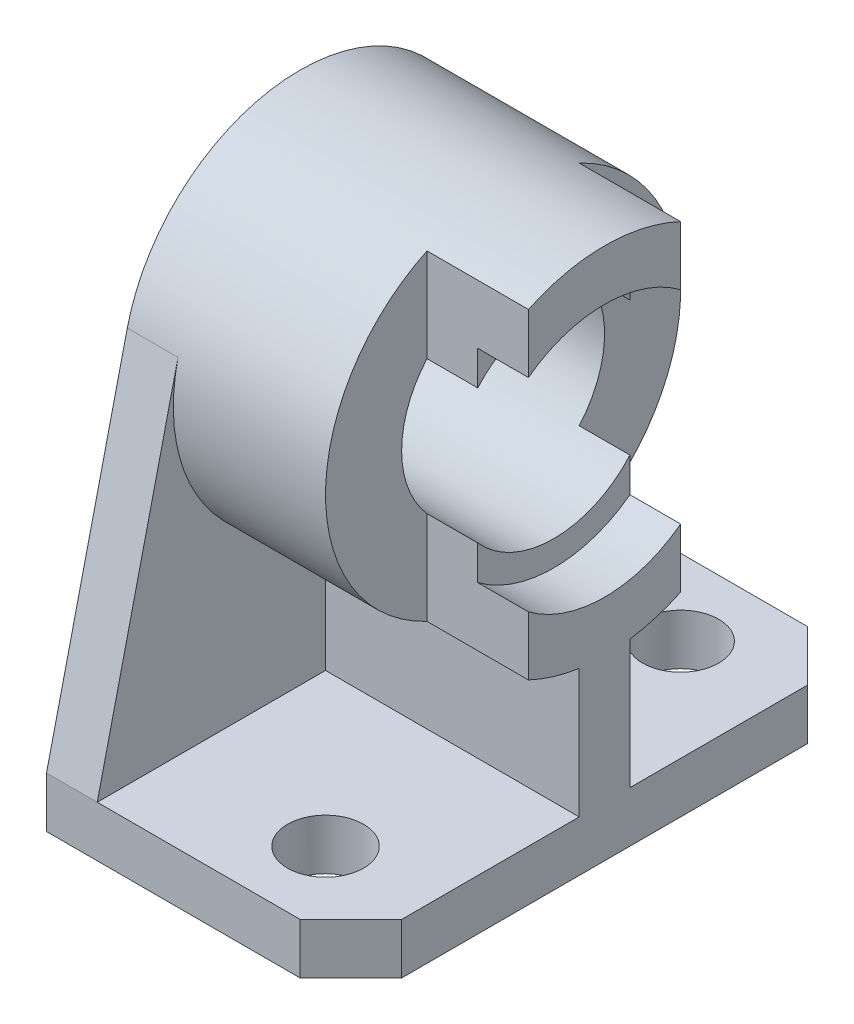
ISO-10303-21;
HEADER;
FILE_DESCRIPTION(('STEP AP214'),'2;1');
FILE_NAME('part.step','',(''),(''),'','','');
FILE_SCHEMA(('AUTOMOTIVE_DESIGN { 1 0 10303 214 1 1 1 1 }'));
ENDSEC;
DATA;
#1=APPLICATION_CONTEXT('core data for automotive mechanical design processes');
#2=APPLICATION_PROTOCOL_DEFINITION('international standard','automotive_design',2000,#1);
#3=PRODUCT_CONTEXT('',#1,'mechanical');
#4=PRODUCT('Part','Part','',(#3));
#5=PRODUCT_RELATED_PRODUCT_CATEGORY('part','',(#4));
#6=PRODUCT_DEFINITION_FORMATION('','',#4);
#7=PRODUCT_DEFINITION_CONTEXT('part definition',#1,'design');
#8=PRODUCT_DEFINITION('design','',#6,#7);
#9=PRODUCT_DEFINITION_SHAPE('','',#8);
#10=(LENGTH_UNIT() NAMED_UNIT(*) SI_UNIT(.MILLI.,.METRE.));
#11=(NAMED_UNIT(*) PLANE_ANGLE_UNIT() SI_UNIT($,.RADIAN.));
#12=(NAMED_UNIT(*) SI_UNIT($,.STERADIAN.) SOLID_ANGLE_UNIT());
#13=UNCERTAINTY_MEASURE_WITH_UNIT(LENGTH_MEASURE(1.E-05),#10,'distance_accuracy_value','');
#14=(GEOMETRIC_REPRESENTATION_CONTEXT(3) GLOBAL_UNCERTAINTY_ASSIGNED_CONTEXT((#13)) GLOBAL_UNIT_ASSIGNED_CONTEXT((#10,
#11,#12)) REPRESENTATION_CONTEXT('',''));
#15=CARTESIAN_POINT('',(0.,0.,0.));
#16=DIRECTION('',(0.,0.,1.));
#17=DIRECTION('',(1.,0.,0.));
#18=AXIS2_PLACEMENT_3D('',#15,#16,#17);
#19=CARTESIAN_POINT('',(60.,-60.,40.));
#20=DIRECTION('',(1.,0.,0.));
#21=DIRECTION('',(0.,0.,-1.));
#22=AXIS2_PLACEMENT_3D('',#19,#20,#21);
#23=PLANE('',#22);
#24=DIRECTION('',(0.,1.,0.));
#25=VECTOR('',#24,1.);
#26=CARTESIAN_POINT('',(60.,31.6227766016838,15.));
#27=LINE('',#26,#25);
#28=CARTESIAN_POINT('',(60.,-31.6227766016838,15.));
#29=VERTEX_POINT('',#28);
#30=CARTESIAN_POINT('',(60.,-20.,15.));
#31=VERTEX_POINT('',#30);
#32=EDGE_CURVE('E216',#29,#31,#27,.T.);
#33=ORIENTED_EDGE('',*,*,#32,.F.);
#34=CARTESIAN_POINT('',(60.,0.,0.));
#35=DIRECTION('',(1.,0.,0.));
#36=DIRECTION('',(0.,0.,-1.));
#37=AXIS2_PLACEMENT_3D('',#34,#35,#36);
#38=CIRCLE('',#37,35.);
#39=CARTESIAN_POINT('',(60.,-34.6410161513775,5.));
#40=VERTEX_POINT('',#39);
#41=EDGE_CURVE('E288',#29,#40,#38,.T.);
#42=ORIENTED_EDGE('',*,*,#41,.T.);
#43=DIRECTION('',(0.,-1.,0.));
#44=VECTOR('',#43,1.);
#45=CARTESIAN_POINT('',(60.,-34.6410161513775,5.));
#46=LINE('',#45,#44);
#47=CARTESIAN_POINT('',(60.,-60.,5.));
#48=VERTEX_POINT('',#47);
#49=EDGE_CURVE('E284',#40,#48,#46,.T.);
#50=ORIENTED_EDGE('',*,*,#49,.T.);
#51=DIRECTION('',(0.,0.,1.));
#52=VECTOR('',#51,1.);
#53=CARTESIAN_POINT('',(60.,-60.,40.));
#54=LINE('',#53,#52);
#55=CARTESIAN_POINT('',(60.,-60.,40.));
#56=VERTEX_POINT('',#55);
#57=EDGE_CURVE('E309',#48,#56,#54,.T.);
#58=ORIENTED_EDGE('',*,*,#57,.T.);
#59=DIRECTION('',(0.,-1.,0.));
#60=VECTOR('',#59,1.);
#61=CARTESIAN_POINT('',(60.,-60.,40.));
#62=LINE('',#61,#60);
#63=CARTESIAN_POINT('',(60.,-70.,40.));
#64=VERTEX_POINT('',#63);
#65=EDGE_CURVE('E334',#56,#64,#62,.T.);
#66=ORIENTED_EDGE('',*,*,#65,.T.);
#67=DIRECTION('',(0.,0.,1.));
#68=VECTOR('',#67,1.);
#69=CARTESIAN_POINT('',(60.,-70.,40.));
#70=LINE('',#69,#68);
#71=CARTESIAN_POINT('',(60.,-70.,-40.));
#72=VERTEX_POINT('',#71);
#73=EDGE_CURVE('E323',#72,#64,#70,.T.);
#74=ORIENTED_EDGE('',*,*,#73,.F.);
#75=DIRECTION('',(0.,-1.,0.));
#76=VECTOR('',#75,1.);
#77=CARTESIAN_POINT('',(60.,-60.,-40.));
#78=LINE('',#77,#76);
#79=CARTESIAN_POINT('',(60.,-60.,-40.));
#80=VERTEX_POINT('',#79);
#81=EDGE_CURVE('E333',#80,#72,#78,.T.);
#82=ORIENTED_EDGE('',*,*,#81,.F.);
#83=CARTESIAN_POINT('',(60.,-60.,-5.));
#84=VERTEX_POINT('',#83);
#85=EDGE_CURVE('E313',#80,#84,#54,.T.);
#86=ORIENTED_EDGE('',*,*,#85,.T.);
#87=DIRECTION('',(0.,1.,0.));
#88=VECTOR('',#87,1.);
#89=CARTESIAN_POINT('',(60.,-34.6410161513775,-5.));
#90=LINE('',#89,#88);
#91=CARTESIAN_POINT('',(60.,-34.6410161513775,-5.00000000000001));
#92=VERTEX_POINT('',#91);
#93=EDGE_CURVE('E292',#84,#92,#90,.T.);
#94=ORIENTED_EDGE('',*,*,#93,.T.);
#95=CARTESIAN_POINT('',(60.,-31.6227766016838,-15.));
#96=VERTEX_POINT('',#95);
#97=EDGE_CURVE('E287',#92,#96,#38,.T.);
#98=ORIENTED_EDGE('',*,*,#97,.T.);
#99=DIRECTION('',(0.,-1.,0.));
#100=VECTOR('',#99,1.);
#101=CARTESIAN_POINT('',(60.,31.6227766016838,-15.));
#102=LINE('',#101,#100);
#103=CARTESIAN_POINT('',(60.,-20.,-15.));
#104=VERTEX_POINT('',#103);
#105=EDGE_CURVE('E416',#104,#96,#102,.T.);
#106=ORIENTED_EDGE('',*,*,#105,.F.);
#107=CARTESIAN_POINT('',(60.,0.,0.));
#108=DIRECTION('',(-1.,0.,0.));
#109=DIRECTION('',(0.,0.,1.));
#110=AXIS2_PLACEMENT_3D('',#107,#108,#109);
#111=CIRCLE('',#110,25.);
#112=EDGE_CURVE('E254',#104,#31,#111,.T.);
#113=ORIENTED_EDGE('',*,*,#112,.T.);
#114=EDGE_LOOP('',(#33,#42,#50,#58,#66,#74,#82,#86,#94,#98,#106,#113));
#115=FACE_BOUND('',#114,.T.);
#116=ADVANCED_FACE('F43',(#115),#23,.T.);
#117=CARTESIAN_POINT('',(0.,0.,0.));
#118=DIRECTION('',(-1.,0.,0.));
#119=DIRECTION('',(0.,0.,1.));
#120=AXIS2_PLACEMENT_3D('',#117,#118,#119);
#121=CYLINDRICAL_SURFACE('',#120,25.);
#122=DIRECTION('',(-1.,0.,0.));
#123=VECTOR('',#122,1.);
#124=CARTESIAN_POINT('',(0.,-20.,15.));
#125=LINE('',#124,#123);
#126=CARTESIAN_POINT('',(50.,-20.,15.));
#127=VERTEX_POINT('',#126);
#128=EDGE_CURVE('E242',#31,#127,#125,.T.);
#129=ORIENTED_EDGE('',*,*,#128,.F.);
#130=ORIENTED_EDGE('',*,*,#112,.F.);
#131=DIRECTION('',(-1.,0.,0.));
#132=VECTOR('',#131,1.);
#133=CARTESIAN_POINT('',(0.,-20.,-15.));
#134=LINE('',#133,#132);
#135=CARTESIAN_POINT('',(50.,-20.,-15.));
#136=VERTEX_POINT('',#135);
#137=EDGE_CURVE('E396',#136,#104,#134,.F.);
#138=ORIENTED_EDGE('',*,*,#137,.F.);
#139=CARTESIAN_POINT('',(50.,0.,0.));
#140=DIRECTION('',(-1.,0.,0.));
#141=DIRECTION('',(0.,0.,1.));
#142=AXIS2_PLACEMENT_3D('',#139,#140,#141);
#143=CIRCLE('',#142,25.);
#144=EDGE_CURVE('E253',#136,#127,#143,.T.);
#145=ORIENTED_EDGE('',*,*,#144,.T.);
#146=EDGE_LOOP('',(#129,#130,#138,#145));
#147=FACE_BOUND('',#146,.T.);
#148=ADVANCED_FACE('F429',(#147),#121,.F.);
#149=CARTESIAN_POINT('',(50.,25.,0.));
#150=DIRECTION('',(1.,0.,0.));
#151=DIRECTION('',(0.,0.,-1.));
#152=AXIS2_PLACEMENT_3D('',#149,#150,#151);
#153=PLANE('',#152);
#154=DIRECTION('',(0.,1.,0.));
#155=VECTOR('',#154,1.);
#156=CARTESIAN_POINT('',(50.,25.,15.));
#157=LINE('',#156,#155);
#158=CARTESIAN_POINT('',(50.,-13.228756555323,15.));
#159=VERTEX_POINT('',#158);
#160=EDGE_CURVE('E237',#127,#159,#157,.T.);
#161=ORIENTED_EDGE('',*,*,#160,.F.);
#162=ORIENTED_EDGE('',*,*,#144,.F.);
#163=DIRECTION('',(0.,-1.,0.));
#164=VECTOR('',#163,1.);
#165=CARTESIAN_POINT('',(50.,25.,-15.));
#166=LINE('',#165,#164);
#167=CARTESIAN_POINT('',(50.,-13.228756555323,-15.));
#168=VERTEX_POINT('',#167);
#169=EDGE_CURVE('E402',#168,#136,#166,.T.);
#170=ORIENTED_EDGE('',*,*,#169,.F.);
#171=CARTESIAN_POINT('',(50.,0.,0.));
#172=DIRECTION('',(-1.,0.,0.));
#173=DIRECTION('',(0.,0.,1.));
#174=AXIS2_PLACEMENT_3D('',#171,#172,#173);
#175=CIRCLE('',#174,20.);
#176=EDGE_CURVE('E249',#168,#159,#175,.T.);
#177=ORIENTED_EDGE('',*,*,#176,.T.);
#178=EDGE_LOOP('',(#161,#162,#170,#177));
#179=FACE_BOUND('',#178,.T.);
#180=ADVANCED_FACE('F452',(#179),#153,.T.);
#181=CARTESIAN_POINT('',(10.,0.,0.));
#182=DIRECTION('',(1.,0.,0.));
#183=DIRECTION('',(0.,0.,-1.));
#184=AXIS2_PLACEMENT_3D('',#181,#182,#183);
#185=PLANE('',#184);
#186=CARTESIAN_POINT('',(10.,0.,0.));
#187=DIRECTION('',(1.,0.,0.));
#188=DIRECTION('',(0.,0.,-1.));
#189=AXIS2_PLACEMENT_3D('',#186,#187,#188);
#190=CIRCLE('',#189,35.);
#191=CARTESIAN_POINT('',(10.,-34.6410161513775,-5.00000000000001));
#192=VERTEX_POINT('',#191);
#193=CARTESIAN_POINT('',(10.,7.981491866062,-34.0777902392744));
#194=VERTEX_POINT('',#193);
#195=EDGE_CURVE('E277',#192,#194,#190,.T.);
#196=ORIENTED_EDGE('',*,*,#195,.F.);
#197=DIRECTION('',(0.,1.,0.));
#198=VECTOR('',#197,1.);
#199=CARTESIAN_POINT('',(10.,-34.6410161513775,-5.));
#200=LINE('',#199,#198);
#201=CARTESIAN_POINT('',(10.,-60.,-5.));
#202=VERTEX_POINT('',#201);
#203=EDGE_CURVE('E276',#202,#192,#200,.T.);
#204=ORIENTED_EDGE('',*,*,#203,.F.);
#205=DIRECTION('',(0.,0.,-1.));
#206=VECTOR('',#205,1.);
#207=CARTESIAN_POINT('',(10.,-60.,50.));
#208=LINE('',#207,#206);
#209=CARTESIAN_POINT('',(10.,-60.,-50.));
#210=VERTEX_POINT('',#209);
#211=EDGE_CURVE('E301',#202,#210,#208,.T.);
#212=ORIENTED_EDGE('',*,*,#211,.T.);
#213=DIRECTION('',(0.,0.973651149693554,0.228042624744629));
#214=VECTOR('',#213,1.);
#215=CARTESIAN_POINT('',(10.,7.981491866062,-34.0777902392744));
#216=LINE('',#215,#214);
#217=EDGE_CURVE('E338',#210,#194,#216,.T.);
#218=ORIENTED_EDGE('',*,*,#217,.T.);
#219=EDGE_LOOP('',(#196,#204,#212,#218));
#220=FACE_BOUND('',#219,.T.);
#221=ADVANCED_FACE('F530',(#220),#185,.T.);
#222=DIRECTION('',(0.,-1.,0.));
#223=VECTOR('',#222,1.);
#224=CARTESIAN_POINT('',(10.,-34.6410161513775,5.));
#225=LINE('',#224,#223);
#226=CARTESIAN_POINT('',(10.,-34.6410161513775,5.));
#227=VERTEX_POINT('',#226);
#228=CARTESIAN_POINT('',(10.,-60.,5.));
#229=VERTEX_POINT('',#228);
#230=EDGE_CURVE('E275',#227,#229,#225,.T.);
#231=ORIENTED_EDGE('',*,*,#230,.F.);
#232=CARTESIAN_POINT('',(10.,7.98149186606201,34.0777902392744));
#233=VERTEX_POINT('',#232);
#234=EDGE_CURVE('E279',#233,#227,#190,.T.);
#235=ORIENTED_EDGE('',*,*,#234,.F.);
#236=DIRECTION('',(0.,-0.973651149693554,0.228042624744629));
#237=VECTOR('',#236,1.);
#238=CARTESIAN_POINT('',(10.,-60.,50.));
#239=LINE('',#238,#237);
#240=CARTESIAN_POINT('',(10.,-60.,50.));
#241=VERTEX_POINT('',#240);
#242=EDGE_CURVE('E344',#233,#241,#239,.T.);
#243=ORIENTED_EDGE('',*,*,#242,.T.);
#244=EDGE_CURVE('E300',#241,#229,#208,.T.);
#245=ORIENTED_EDGE('',*,*,#244,.T.);
#246=EDGE_LOOP('',(#231,#235,#243,#245));
#247=FACE_BOUND('',#246,.T.);
#248=ADVANCED_FACE('F487',(#247),#185,.T.);
#249=CARTESIAN_POINT('',(0.,-60.,0.));
#250=DIRECTION('',(0.,-1.,0.));
#251=DIRECTION('',(0.,0.,-1.));
#252=AXIS2_PLACEMENT_3D('',#249,#250,#251);
#253=PLANE('',#252);
#254=CARTESIAN_POINT('',(40.,-60.,-35.));
#255=DIRECTION('',(0.,1.,0.));
#256=DIRECTION('',(0.,0.,1.));
#257=AXIS2_PLACEMENT_3D('',#254,#255,#256);
#258=CIRCLE('',#257,7.5);
#259=CARTESIAN_POINT('',(40.,-60.,-27.5));
#260=VERTEX_POINT('',#259);
#261=EDGE_CURVE('E257',#260,#260,#258,.T.);
#262=ORIENTED_EDGE('',*,*,#261,.F.);
#263=EDGE_LOOP('',(#262));
#264=FACE_BOUND('',#263,.T.);
#265=DIRECTION('',(-1.,0.,0.));
#266=VECTOR('',#265,1.);
#267=CARTESIAN_POINT('',(178.004237212059,-60.,-5.));
#268=LINE('',#267,#266);
#269=EDGE_CURVE('E270',#84,#202,#268,.T.);
#270=ORIENTED_EDGE('',*,*,#269,.F.);
#271=ORIENTED_EDGE('',*,*,#85,.F.);
#272=DIRECTION('',(0.707106781186548,0.,0.707106781186547));
#273=VECTOR('',#272,1.);
#274=CARTESIAN_POINT('',(50.,-60.,-50.));
#275=LINE('',#274,#273);
#276=CARTESIAN_POINT('',(50.,-60.,-50.));
#277=VERTEX_POINT('',#276);
#278=EDGE_CURVE('E307',#277,#80,#275,.T.);
#279=ORIENTED_EDGE('',*,*,#278,.F.);
#280=DIRECTION('',(1.,0.,0.));
#281=VECTOR('',#280,1.);
#282=CARTESIAN_POINT('',(10.,-60.,-50.));
#283=LINE('',#282,#281);
#284=EDGE_CURVE('E305',#210,#277,#283,.T.);
#285=ORIENTED_EDGE('',*,*,#284,.F.);
#286=ORIENTED_EDGE('',*,*,#211,.F.);
#287=EDGE_LOOP('',(#270,#271,#279,#285,#286));
#288=FACE_BOUND('',#287,.T.);
#289=ADVANCED_FACE('F484',(#264,#288),#253,.F.);
#290=CARTESIAN_POINT('',(40.,-60.,35.));
#291=DIRECTION('',(0.,1.,0.));
#292=DIRECTION('',(0.,0.,-1.));
#293=AXIS2_PLACEMENT_3D('',#290,#291,#292);
#294=CIRCLE('',#293,7.5);
#295=CARTESIAN_POINT('',(40.,-60.,27.5));
#296=VERTEX_POINT('',#295);
#297=EDGE_CURVE('E259',#296,#296,#294,.T.);
#298=ORIENTED_EDGE('',*,*,#297,.F.);
#299=EDGE_LOOP('',(#298));
#300=FACE_BOUND('',#299,.T.);
#301=DIRECTION('',(-1.,0.,0.));
#302=VECTOR('',#301,1.);
#303=CARTESIAN_POINT('',(178.004237212059,-60.,5.));
#304=LINE('',#303,#302);
#305=EDGE_CURVE('E273',#48,#229,#304,.T.);
#306=ORIENTED_EDGE('',*,*,#305,.T.);
#307=ORIENTED_EDGE('',*,*,#244,.F.);
#308=DIRECTION('',(-1.,0.,0.));
#309=VECTOR('',#308,1.);
#310=CARTESIAN_POINT('',(10.,-60.,50.));
#311=LINE('',#310,#309);
#312=CARTESIAN_POINT('',(50.,-60.,50.));
#313=VERTEX_POINT('',#312);
#314=EDGE_CURVE('E320',#313,#241,#311,.T.);
#315=ORIENTED_EDGE('',*,*,#314,.F.);
#316=DIRECTION('',(-0.707106781186547,0.,0.707106781186548));
#317=VECTOR('',#316,1.);
#318=CARTESIAN_POINT('',(50.,-60.,50.));
#319=LINE('',#318,#317);
#320=EDGE_CURVE('E314',#56,#313,#319,.T.);
#321=ORIENTED_EDGE('',*,*,#320,.F.);
#322=ORIENTED_EDGE('',*,*,#57,.F.);
#323=EDGE_LOOP('',(#306,#307,#315,#321,#322));
#324=FACE_BOUND('',#323,.T.);
#325=ADVANCED_FACE('F488',(#300,#324),#253,.F.);
#326=CARTESIAN_POINT('',(10.,-70.,50.));
#327=DIRECTION('',(0.,0.,-1.));
#328=DIRECTION('',(-1.,0.,0.));
#329=AXIS2_PLACEMENT_3D('',#326,#327,#328);
#330=PLANE('',#329);
#331=DIRECTION('',(0.,-1.,0.));
#332=VECTOR('',#331,1.);
#333=CARTESIAN_POINT('',(0.,-70.,50.));
#334=LINE('',#333,#332);
#335=CARTESIAN_POINT('',(0.,-60.,50.));
#336=VERTEX_POINT('',#335);
#337=CARTESIAN_POINT('',(0.,-70.,50.));
#338=VERTEX_POINT('',#337);
#339=EDGE_CURVE('E335',#336,#338,#334,.T.);
#340=ORIENTED_EDGE('',*,*,#339,.T.);
#341=DIRECTION('',(-1.,0.,0.));
#342=VECTOR('',#341,1.);
#343=CARTESIAN_POINT('',(10.,-70.,50.));
#344=LINE('',#343,#342);
#345=CARTESIAN_POINT('',(50.,-70.,50.));
#346=VERTEX_POINT('',#345);
#347=EDGE_CURVE('E375',#346,#338,#344,.T.);
#348=ORIENTED_EDGE('',*,*,#347,.F.);
#349=DIRECTION('',(0.,-1.,0.));
#350=VECTOR('',#349,1.);
#351=CARTESIAN_POINT('',(50.,-60.,50.));
#352=LINE('',#351,#350);
#353=EDGE_CURVE('E328',#313,#346,#352,.T.);
#354=ORIENTED_EDGE('',*,*,#353,.F.);
#355=ORIENTED_EDGE('',*,*,#314,.T.);
#356=DIRECTION('',(-1.,0.,0.));
#357=VECTOR('',#356,1.);
#358=CARTESIAN_POINT('',(10.,-60.,50.));
#359=LINE('',#358,#357);
#360=EDGE_CURVE('E347',#241,#336,#359,.T.);
#361=ORIENTED_EDGE('',*,*,#360,.T.);
#362=EDGE_LOOP('',(#340,#348,#354,#355,#361));
#363=FACE_BOUND('',#362,.T.);
#364=ADVANCED_FACE('F44',(#363),#330,.F.);
#365=CARTESIAN_POINT('',(10.,-70.,50.));
#366=DIRECTION('',(0.,1.,0.));
#367=DIRECTION('',(0.,0.,1.));
#368=AXIS2_PLACEMENT_3D('',#365,#366,#367);
#369=PLANE('',#368);
#370=CARTESIAN_POINT('',(40.,-70.,-35.));
#371=DIRECTION('',(0.,1.,0.));
#372=DIRECTION('',(0.,0.,1.));
#373=AXIS2_PLACEMENT_3D('',#370,#371,#372);
#374=CIRCLE('',#373,7.5);
#375=CARTESIAN_POINT('',(40.,-70.,-27.5));
#376=VERTEX_POINT('',#375);
#377=EDGE_CURVE('E263',#376,#376,#374,.F.);
#378=ORIENTED_EDGE('',*,*,#377,.F.);
#379=EDGE_LOOP('',(#378));
#380=FACE_BOUND('',#379,.T.);
#381=CARTESIAN_POINT('',(40.,-70.,35.));
#382=DIRECTION('',(0.,1.,0.));
#383=DIRECTION('',(0.,0.,1.));
#384=AXIS2_PLACEMENT_3D('',#381,#382,#383);
#385=CIRCLE('',#384,7.5);
#386=CARTESIAN_POINT('',(40.,-70.,42.5));
#387=VERTEX_POINT('',#386);
#388=EDGE_CURVE('E262',#387,#387,#385,.F.);
#389=ORIENTED_EDGE('',*,*,#388,.F.);
#390=EDGE_LOOP('',(#389));
#391=FACE_BOUND('',#390,.T.);
#392=DIRECTION('',(0.,0.,-1.));
#393=VECTOR('',#392,1.);
#394=CARTESIAN_POINT('',(0.,-70.,50.));
#395=LINE('',#394,#393);
#396=CARTESIAN_POINT('',(0.,-70.,-50.));
#397=VERTEX_POINT('',#396);
#398=EDGE_CURVE('E349',#338,#397,#395,.T.);
#399=ORIENTED_EDGE('',*,*,#398,.T.);
#400=DIRECTION('',(-1.,0.,0.));
#401=VECTOR('',#400,1.);
#402=CARTESIAN_POINT('',(10.,-70.,-50.));
#403=LINE('',#402,#401);
#404=CARTESIAN_POINT('',(50.,-70.,-50.));
#405=VERTEX_POINT('',#404);
#406=EDGE_CURVE('E369',#405,#397,#403,.T.);
#407=ORIENTED_EDGE('',*,*,#406,.F.);
#408=DIRECTION('',(0.707106781186548,0.,0.707106781186547));
#409=VECTOR('',#408,1.);
#410=CARTESIAN_POINT('',(50.,-70.,-50.));
#411=LINE('',#410,#409);
#412=EDGE_CURVE('E285',#405,#72,#411,.T.);
#413=ORIENTED_EDGE('',*,*,#412,.T.);
#414=ORIENTED_EDGE('',*,*,#73,.T.);
#415=DIRECTION('',(-0.707106781186547,0.,0.707106781186548));
#416=VECTOR('',#415,1.);
#417=CARTESIAN_POINT('',(50.,-70.,50.));
#418=LINE('',#417,#416);
#419=EDGE_CURVE('E326',#64,#346,#418,.T.);
#420=ORIENTED_EDGE('',*,*,#419,.T.);
#421=ORIENTED_EDGE('',*,*,#347,.T.);
#422=EDGE_LOOP('',(#399,#407,#413,#414,#420,#421));
#423=FACE_BOUND('',#422,.T.);
#424=ADVANCED_FACE('F509',(#380,#391,#423),#369,.F.);
#425=CARTESIAN_POINT('',(10.,-60.,-50.));
#426=DIRECTION('',(0.,0.,1.));
#427=DIRECTION('',(1.,0.,0.));
#428=AXIS2_PLACEMENT_3D('',#425,#426,#427);
#429=PLANE('',#428);
#430=DIRECTION('',(0.,1.,0.));
#431=VECTOR('',#430,1.);
#432=CARTESIAN_POINT('',(0.,-60.,-50.));
#433=LINE('',#432,#431);
#434=CARTESIAN_POINT('',(0.,-60.,-50.));
#435=VERTEX_POINT('',#434);
#436=EDGE_CURVE('E351',#397,#435,#433,.T.);
#437=ORIENTED_EDGE('',*,*,#436,.T.);
#438=DIRECTION('',(-1.,0.,0.));
#439=VECTOR('',#438,1.);
#440=CARTESIAN_POINT('',(10.,-60.,-50.));
#441=LINE('',#440,#439);
#442=EDGE_CURVE('E368',#210,#435,#441,.T.);
#443=ORIENTED_EDGE('',*,*,#442,.F.);
#444=ORIENTED_EDGE('',*,*,#284,.T.);
#445=DIRECTION('',(0.,-1.,0.));
#446=VECTOR('',#445,1.);
#447=CARTESIAN_POINT('',(50.,-60.,-50.));
#448=LINE('',#447,#446);
#449=EDGE_CURVE('E319',#277,#405,#448,.T.);
#450=ORIENTED_EDGE('',*,*,#449,.T.);
#451=ORIENTED_EDGE('',*,*,#406,.T.);
#452=EDGE_LOOP('',(#437,#443,#444,#450,#451));
#453=FACE_BOUND('',#452,.T.);
#454=ADVANCED_FACE('F508',(#453),#429,.F.);
#455=CARTESIAN_POINT('',(10.,7.981491866062,-34.0777902392744));
#456=DIRECTION('',(0.,-0.228042624744629,0.973651149693554));
#457=DIRECTION('',(0.,-0.973651149693554,-0.228042624744629));
#458=AXIS2_PLACEMENT_3D('',#455,#456,#457);
#459=PLANE('',#458);
#460=DIRECTION('',(0.,0.973651149693554,0.228042624744629));
#461=VECTOR('',#460,1.);
#462=CARTESIAN_POINT('',(0.,7.981491866062,-34.0777902392744));
#463=LINE('',#462,#461);
#464=CARTESIAN_POINT('',(0.,7.981491866062,-34.0777902392744));
#465=VERTEX_POINT('',#464);
#466=EDGE_CURVE('E354',#435,#465,#463,.T.);
#467=ORIENTED_EDGE('',*,*,#466,.T.);
#468=DIRECTION('',(-1.,0.,0.));
#469=VECTOR('',#468,1.);
#470=CARTESIAN_POINT('',(10.,7.981491866062,-34.0777902392744));
#471=LINE('',#470,#469);
#472=EDGE_CURVE('E361',#194,#465,#471,.T.);
#473=ORIENTED_EDGE('',*,*,#472,.F.);
#474=ORIENTED_EDGE('',*,*,#217,.F.);
#475=ORIENTED_EDGE('',*,*,#442,.T.);
#476=EDGE_LOOP('',(#467,#473,#474,#475));
#477=FACE_BOUND('',#476,.T.);
#478=ADVANCED_FACE('F525',(#477),#459,.F.);
#479=CARTESIAN_POINT('',(10.,0.,0.));
#480=DIRECTION('',(-1.,0.,0.));
#481=DIRECTION('',(0.,0.,1.));
#482=AXIS2_PLACEMENT_3D('',#479,#480,#481);
#483=CYLINDRICAL_SURFACE('',#482,35.);
#484=ORIENTED_EDGE('',*,*,#41,.F.);
#485=DIRECTION('',(1.,0.,0.));
#486=VECTOR('',#485,1.);
#487=CARTESIAN_POINT('',(40.,-31.6227766016838,15.));
#488=LINE('',#487,#486);
#489=CARTESIAN_POINT('',(40.,-31.6227766016838,15.));
#490=VERTEX_POINT('',#489);
#491=EDGE_CURVE('E226',#490,#29,#488,.T.);
#492=ORIENTED_EDGE('',*,*,#491,.F.);
#493=CARTESIAN_POINT('',(40.,0.,0.));
#494=DIRECTION('',(-1.,0.,0.));
#495=DIRECTION('',(0.,0.,1.));
#496=AXIS2_PLACEMENT_3D('',#493,#494,#495);
#497=CIRCLE('',#496,35.);
#498=CARTESIAN_POINT('',(40.,31.6227766016838,15.));
#499=VERTEX_POINT('',#498);
#500=EDGE_CURVE('E211',#490,#499,#497,.T.);
#501=ORIENTED_EDGE('',*,*,#500,.T.);
#502=DIRECTION('',(1.,0.,0.));
#503=VECTOR('',#502,1.);
#504=CARTESIAN_POINT('',(40.,31.6227766016838,15.));
#505=LINE('',#504,#503);
#506=CARTESIAN_POINT('',(60.,31.6227766016838,15.));
#507=VERTEX_POINT('',#506);
#508=EDGE_CURVE('E218',#499,#507,#505,.T.);
#509=ORIENTED_EDGE('',*,*,#508,.T.);
#510=CARTESIAN_POINT('',(60.,31.6227766016838,-15.));
#511=VERTEX_POINT('',#510);
#512=EDGE_CURVE('E286',#511,#507,#38,.T.);
#513=ORIENTED_EDGE('',*,*,#512,.F.);
#514=DIRECTION('',(1.,0.,0.));
#515=VECTOR('',#514,1.);
#516=CARTESIAN_POINT('',(40.,31.6227766016838,-15.));
#517=LINE('',#516,#515);
#518=CARTESIAN_POINT('',(40.,31.6227766016838,-15.));
#519=VERTEX_POINT('',#518);
#520=EDGE_CURVE('E415',#519,#511,#517,.T.);
#521=ORIENTED_EDGE('',*,*,#520,.F.);
#522=CARTESIAN_POINT('',(40.,0.,0.));
#523=DIRECTION('',(1.,0.,0.));
#524=DIRECTION('',(0.,0.,-1.));
#525=AXIS2_PLACEMENT_3D('',#522,#523,#524);
#526=CIRCLE('',#525,35.);
#527=CARTESIAN_POINT('',(40.,-31.6227766016838,-15.));
#528=VERTEX_POINT('',#527);
#529=EDGE_CURVE('E401',#528,#519,#526,.T.);
#530=ORIENTED_EDGE('',*,*,#529,.F.);
#531=DIRECTION('',(1.,0.,0.));
#532=VECTOR('',#531,1.);
#533=CARTESIAN_POINT('',(40.,-31.6227766016838,-15.));
#534=LINE('',#533,#532);
#535=EDGE_CURVE('E410',#528,#96,#534,.T.);
#536=ORIENTED_EDGE('',*,*,#535,.T.);
#537=ORIENTED_EDGE('',*,*,#97,.F.);
#538=DIRECTION('',(-1.,0.,0.));
#539=VECTOR('',#538,1.);
#540=CARTESIAN_POINT('',(178.004237212059,-34.6410161513775,-5.00000000000001));
#541=LINE('',#540,#539);
#542=EDGE_CURVE('E282',#92,#192,#541,.T.);
#543=ORIENTED_EDGE('',*,*,#542,.T.);
#544=ORIENTED_EDGE('',*,*,#195,.T.);
#545=ORIENTED_EDGE('',*,*,#472,.T.);
#546=CARTESIAN_POINT('',(0.,0.,0.));
#547=DIRECTION('',(1.,0.,0.));
#548=DIRECTION('',(0.,0.,-1.));
#549=AXIS2_PLACEMENT_3D('',#546,#547,#548);
#550=CIRCLE('',#549,35.);
#551=CARTESIAN_POINT('',(0.,7.98149186606201,34.0777902392744));
#552=VERTEX_POINT('',#551);
#553=EDGE_CURVE('E355',#465,#552,#550,.T.);
#554=ORIENTED_EDGE('',*,*,#553,.T.);
#555=DIRECTION('',(-1.,0.,0.));
#556=VECTOR('',#555,1.);
#557=CARTESIAN_POINT('',(10.,7.98149186606201,34.0777902392744));
#558=LINE('',#557,#556);
#559=EDGE_CURVE('E358',#233,#552,#558,.T.);
#560=ORIENTED_EDGE('',*,*,#559,.F.);
#561=ORIENTED_EDGE('',*,*,#234,.T.);
#562=DIRECTION('',(-1.,0.,0.));
#563=VECTOR('',#562,1.);
#564=CARTESIAN_POINT('',(178.004237212059,-34.6410161513775,5.));
#565=LINE('',#564,#563);
#566=EDGE_CURVE('E274',#40,#227,#565,.T.);
#567=ORIENTED_EDGE('',*,*,#566,.F.);
#568=EDGE_LOOP('',(#484,#492,#501,#509,#513,#521,#530,#536,#537,#543,#544,#545,#554,#560,#561,#567));
#569=FACE_BOUND('',#568,.T.);
#570=ADVANCED_FACE('F230',(#569),#483,.T.);
#571=CARTESIAN_POINT('',(10.,-60.,50.));
#572=DIRECTION('',(0.,-0.228042624744629,-0.973651149693554));
#573=DIRECTION('',(0.,0.973651149693554,-0.228042624744629));
#574=AXIS2_PLACEMENT_3D('',#571,#572,#573);
#575=PLANE('',#574);
#576=DIRECTION('',(0.,-0.973651149693554,0.228042624744629));
#577=VECTOR('',#576,1.);
#578=CARTESIAN_POINT('',(0.,-60.,50.));
#579=LINE('',#578,#577);
#580=EDGE_CURVE('E345',#552,#336,#579,.T.);
#581=ORIENTED_EDGE('',*,*,#580,.T.);
#582=ORIENTED_EDGE('',*,*,#360,.F.);
#583=ORIENTED_EDGE('',*,*,#242,.F.);
#584=ORIENTED_EDGE('',*,*,#559,.T.);
#585=EDGE_LOOP('',(#581,#582,#583,#584));
#586=FACE_BOUND('',#585,.T.);
#587=ADVANCED_FACE('F477',(#586),#575,.F.);
#588=CARTESIAN_POINT('',(0.,0.,0.));
#589=DIRECTION('',(1.,0.,0.));
#590=DIRECTION('',(0.,0.,-1.));
#591=AXIS2_PLACEMENT_3D('',#588,#589,#590);
#592=PLANE('',#591);
#593=CARTESIAN_POINT('',(0.,0.,0.));
#594=DIRECTION('',(-1.,0.,0.));
#595=DIRECTION('',(0.,0.,1.));
#596=AXIS2_PLACEMENT_3D('',#593,#594,#595);
#597=CIRCLE('',#596,20.);
#598=CARTESIAN_POINT('',(0.,0.,20.));
#599=VERTEX_POINT('',#598);
#600=EDGE_CURVE('E243',#599,#599,#597,.T.);
#601=ORIENTED_EDGE('',*,*,#600,.F.);
#602=EDGE_LOOP('',(#601));
#603=FACE_BOUND('',#602,.T.);
#604=ORIENTED_EDGE('',*,*,#339,.F.);
#605=ORIENTED_EDGE('',*,*,#580,.F.);
#606=ORIENTED_EDGE('',*,*,#553,.F.);
#607=ORIENTED_EDGE('',*,*,#466,.F.);
#608=ORIENTED_EDGE('',*,*,#436,.F.);
#609=ORIENTED_EDGE('',*,*,#398,.F.);
#610=EDGE_LOOP('',(#604,#605,#606,#607,#608,#609));
#611=FACE_BOUND('',#610,.T.);
#612=ADVANCED_FACE('F474',(#603,#611),#592,.F.);
#613=CARTESIAN_POINT('',(50.,-60.,50.));
#614=DIRECTION('',(0.707106781186548,0.,0.707106781186547));
#615=DIRECTION('',(0.707106781186547,0.,-0.707106781186548));
#616=AXIS2_PLACEMENT_3D('',#613,#614,#615);
#617=PLANE('',#616);
#618=ORIENTED_EDGE('',*,*,#419,.F.);
#619=ORIENTED_EDGE('',*,*,#65,.F.);
#620=ORIENTED_EDGE('',*,*,#320,.T.);
#621=ORIENTED_EDGE('',*,*,#353,.T.);
#622=EDGE_LOOP('',(#618,#619,#620,#621));
#623=FACE_BOUND('',#622,.T.);
#624=ADVANCED_FACE('F467',(#623),#617,.T.);
#625=CARTESIAN_POINT('',(60.,20.,15.));
#626=VERTEX_POINT('',#625);
#627=EDGE_CURVE('E225',#626,#507,#27,.T.);
#628=ORIENTED_EDGE('',*,*,#627,.F.);
#629=CARTESIAN_POINT('',(60.,20.,-15.));
#630=VERTEX_POINT('',#629);
#631=EDGE_CURVE('E258',#626,#630,#111,.T.);
#632=ORIENTED_EDGE('',*,*,#631,.T.);
#633=EDGE_CURVE('E413',#511,#630,#102,.T.);
#634=ORIENTED_EDGE('',*,*,#633,.F.);
#635=ORIENTED_EDGE('',*,*,#512,.T.);
#636=EDGE_LOOP('',(#628,#632,#634,#635));
#637=FACE_BOUND('',#636,.T.);
#638=ADVANCED_FACE('F438',(#637),#23,.T.);
#639=CARTESIAN_POINT('',(50.,-60.,-50.));
#640=DIRECTION('',(0.707106781186547,0.,-0.707106781186548));
#641=DIRECTION('',(-0.707106781186548,0.,-0.707106781186547));
#642=AXIS2_PLACEMENT_3D('',#639,#640,#641);
#643=PLANE('',#642);
#644=ORIENTED_EDGE('',*,*,#412,.F.);
#645=ORIENTED_EDGE('',*,*,#449,.F.);
#646=ORIENTED_EDGE('',*,*,#278,.T.);
#647=ORIENTED_EDGE('',*,*,#81,.T.);
#648=EDGE_LOOP('',(#644,#645,#646,#647));
#649=FACE_BOUND('',#648,.T.);
#650=ADVANCED_FACE('F465',(#649),#643,.T.);
#651=CARTESIAN_POINT('',(178.004237212059,-34.6410161513775,-5.));
#652=DIRECTION('',(0.,0.,1.));
#653=DIRECTION('',(0.,-1.,0.));
#654=AXIS2_PLACEMENT_3D('',#651,#652,#653);
#655=PLANE('',#654);
#656=ORIENTED_EDGE('',*,*,#93,.F.);
#657=ORIENTED_EDGE('',*,*,#269,.T.);
#658=ORIENTED_EDGE('',*,*,#203,.T.);
#659=ORIENTED_EDGE('',*,*,#542,.F.);
#660=EDGE_LOOP('',(#656,#657,#658,#659));
#661=FACE_BOUND('',#660,.T.);
#662=ADVANCED_FACE('F472',(#661),#655,.F.);
#663=CARTESIAN_POINT('',(178.004237212059,-34.6410161513775,5.));
#664=DIRECTION('',(0.,0.,-1.));
#665=DIRECTION('',(0.,1.,0.));
#666=AXIS2_PLACEMENT_3D('',#663,#664,#665);
#667=PLANE('',#666);
#668=ORIENTED_EDGE('',*,*,#49,.F.);
#669=ORIENTED_EDGE('',*,*,#566,.T.);
#670=ORIENTED_EDGE('',*,*,#230,.T.);
#671=ORIENTED_EDGE('',*,*,#305,.F.);
#672=EDGE_LOOP('',(#668,#669,#670,#671));
#673=FACE_BOUND('',#672,.T.);
#674=ADVANCED_FACE('F492',(#673),#667,.F.);
#675=CARTESIAN_POINT('',(40.,-70.001,35.));
#676=DIRECTION('',(0.,1.,0.));
#677=DIRECTION('',(0.,0.,1.));
#678=AXIS2_PLACEMENT_3D('',#675,#676,#677);
#679=CYLINDRICAL_SURFACE('',#678,7.5);
#680=ORIENTED_EDGE('',*,*,#297,.T.);
#681=EDGE_LOOP('',(#680));
#682=FACE_BOUND('',#681,.T.);
#683=ORIENTED_EDGE('',*,*,#388,.T.);
#684=EDGE_LOOP('',(#683));
#685=FACE_BOUND('',#684,.T.);
#686=ADVANCED_FACE('F454',(#682,#685),#679,.F.);
#687=CARTESIAN_POINT('',(40.,-70.001,-35.));
#688=DIRECTION('',(0.,1.,0.));
#689=DIRECTION('',(0.,0.,1.));
#690=AXIS2_PLACEMENT_3D('',#687,#688,#689);
#691=CYLINDRICAL_SURFACE('',#690,7.5);
#692=ORIENTED_EDGE('',*,*,#261,.T.);
#693=EDGE_LOOP('',(#692));
#694=FACE_BOUND('',#693,.T.);
#695=ORIENTED_EDGE('',*,*,#377,.T.);
#696=EDGE_LOOP('',(#695));
#697=FACE_BOUND('',#696,.T.);
#698=ADVANCED_FACE('F441',(#694,#697),#691,.F.);
#699=DIRECTION('',(-1.,0.,0.));
#700=VECTOR('',#699,1.);
#701=CARTESIAN_POINT('',(0.,20.,15.));
#702=LINE('',#701,#700);
#703=CARTESIAN_POINT('',(50.,20.,15.));
#704=VERTEX_POINT('',#703);
#705=EDGE_CURVE('E231',#704,#626,#702,.F.);
#706=ORIENTED_EDGE('',*,*,#705,.F.);
#707=CARTESIAN_POINT('',(50.,20.,-15.));
#708=VERTEX_POINT('',#707);
#709=EDGE_CURVE('E252',#704,#708,#143,.T.);
#710=ORIENTED_EDGE('',*,*,#709,.T.);
#711=DIRECTION('',(-1.,0.,0.));
#712=VECTOR('',#711,1.);
#713=CARTESIAN_POINT('',(0.,20.,-15.));
#714=LINE('',#713,#712);
#715=EDGE_CURVE('E234',#630,#708,#714,.T.);
#716=ORIENTED_EDGE('',*,*,#715,.F.);
#717=ORIENTED_EDGE('',*,*,#631,.F.);
#718=EDGE_LOOP('',(#706,#710,#716,#717));
#719=FACE_BOUND('',#718,.T.);
#720=ADVANCED_FACE('F445',(#719),#121,.F.);
#721=CARTESIAN_POINT('',(50.,13.228756555323,15.));
#722=VERTEX_POINT('',#721);
#723=EDGE_CURVE('E232',#722,#704,#157,.T.);
#724=ORIENTED_EDGE('',*,*,#723,.F.);
#725=CARTESIAN_POINT('',(50.,13.228756555323,-15.));
#726=VERTEX_POINT('',#725);
#727=EDGE_CURVE('E250',#722,#726,#175,.T.);
#728=ORIENTED_EDGE('',*,*,#727,.T.);
#729=EDGE_CURVE('E240',#708,#726,#166,.T.);
#730=ORIENTED_EDGE('',*,*,#729,.F.);
#731=ORIENTED_EDGE('',*,*,#709,.F.);
#732=EDGE_LOOP('',(#724,#728,#730,#731));
#733=FACE_BOUND('',#732,.T.);
#734=ADVANCED_FACE('F389',(#733),#153,.T.);
#735=CARTESIAN_POINT('',(0.,0.,0.));
#736=DIRECTION('',(-1.,0.,0.));
#737=DIRECTION('',(0.,0.,1.));
#738=AXIS2_PLACEMENT_3D('',#735,#736,#737);
#739=CYLINDRICAL_SURFACE('',#738,20.);
#740=DIRECTION('',(-1.,0.,0.));
#741=VECTOR('',#740,1.);
#742=CARTESIAN_POINT('',(0.,-13.228756555323,15.));
#743=LINE('',#742,#741);
#744=CARTESIAN_POINT('',(40.,-13.2287565553229,15.));
#745=VERTEX_POINT('',#744);
#746=EDGE_CURVE('E11',#159,#745,#743,.T.);
#747=ORIENTED_EDGE('',*,*,#746,.F.);
#748=ORIENTED_EDGE('',*,*,#176,.F.);
#749=DIRECTION('',(-1.,0.,0.));
#750=VECTOR('',#749,1.);
#751=CARTESIAN_POINT('',(0.,-13.228756555323,-15.));
#752=LINE('',#751,#750);
#753=CARTESIAN_POINT('',(40.,-13.228756555323,-15.));
#754=VERTEX_POINT('',#753);
#755=EDGE_CURVE('E378',#754,#168,#752,.F.);
#756=ORIENTED_EDGE('',*,*,#755,.F.);
#757=CARTESIAN_POINT('',(40.,0.,0.));
#758=DIRECTION('',(1.,0.,0.));
#759=DIRECTION('',(0.,0.,-1.));
#760=AXIS2_PLACEMENT_3D('',#757,#758,#759);
#761=CIRCLE('',#760,20.);
#762=CARTESIAN_POINT('',(40.,13.228756555323,-15.));
#763=VERTEX_POINT('',#762);
#764=EDGE_CURVE('E374',#754,#763,#761,.T.);
#765=ORIENTED_EDGE('',*,*,#764,.T.);
#766=DIRECTION('',(-1.,0.,0.));
#767=VECTOR('',#766,1.);
#768=CARTESIAN_POINT('',(0.,13.228756555323,-15.));
#769=LINE('',#768,#767);
#770=EDGE_CURVE('E379',#726,#763,#769,.T.);
#771=ORIENTED_EDGE('',*,*,#770,.F.);
#772=ORIENTED_EDGE('',*,*,#727,.F.);
#773=DIRECTION('',(-1.,0.,0.));
#774=VECTOR('',#773,1.);
#775=CARTESIAN_POINT('',(0.,13.228756555323,15.));
#776=LINE('',#775,#774);
#777=CARTESIAN_POINT('',(40.,13.2287565553229,15.));
#778=VERTEX_POINT('',#777);
#779=EDGE_CURVE('E51',#778,#722,#776,.F.);
#780=ORIENTED_EDGE('',*,*,#779,.F.);
#781=CARTESIAN_POINT('',(40.,0.,0.));
#782=DIRECTION('',(-1.,0.,0.));
#783=DIRECTION('',(0.,0.,1.));
#784=AXIS2_PLACEMENT_3D('',#781,#782,#783);
#785=CIRCLE('',#784,20.);
#786=EDGE_CURVE('E213',#745,#778,#785,.T.);
#787=ORIENTED_EDGE('',*,*,#786,.F.);
#788=EDGE_LOOP('',(#747,#748,#756,#765,#771,#772,#780,#787));
#789=FACE_BOUND('',#788,.T.);
#790=ORIENTED_EDGE('',*,*,#600,.T.);
#791=EDGE_LOOP('',(#790));
#792=FACE_BOUND('',#791,.T.);
#793=ADVANCED_FACE('F392',(#789,#792),#739,.F.);
#794=CARTESIAN_POINT('',(40.,31.6227766016838,-15.));
#795=DIRECTION('',(0.,0.,1.));
#796=DIRECTION('',(1.,0.,0.));
#797=AXIS2_PLACEMENT_3D('',#794,#795,#796);
#798=PLANE('',#797);
#799=ORIENTED_EDGE('',*,*,#715,.T.);
#800=ORIENTED_EDGE('',*,*,#729,.T.);
#801=ORIENTED_EDGE('',*,*,#770,.T.);
#802=DIRECTION('',(0.,-1.,0.));
#803=VECTOR('',#802,1.);
#804=CARTESIAN_POINT('',(40.,31.6227766016838,-15.));
#805=LINE('',#804,#803);
#806=EDGE_CURVE('E65',#519,#763,#805,.T.);
#807=ORIENTED_EDGE('',*,*,#806,.F.);
#808=ORIENTED_EDGE('',*,*,#520,.T.);
#809=ORIENTED_EDGE('',*,*,#633,.T.);
#810=EDGE_LOOP('',(#799,#800,#801,#807,#808,#809));
#811=FACE_BOUND('',#810,.T.);
#812=ADVANCED_FACE('F397',(#811),#798,.F.);
#813=CARTESIAN_POINT('',(40.,0.,0.));
#814=DIRECTION('',(1.,0.,0.));
#815=DIRECTION('',(0.,0.,-1.));
#816=AXIS2_PLACEMENT_3D('',#813,#814,#815);
#817=PLANE('',#816);
#818=ORIENTED_EDGE('',*,*,#529,.T.);
#819=ORIENTED_EDGE('',*,*,#806,.T.);
#820=ORIENTED_EDGE('',*,*,#764,.F.);
#821=EDGE_CURVE('E417',#754,#528,#805,.T.);
#822=ORIENTED_EDGE('',*,*,#821,.T.);
#823=EDGE_LOOP('',(#818,#819,#820,#822));
#824=FACE_BOUND('',#823,.T.);
#825=ADVANCED_FACE('F659',(#824),#817,.T.);
#826=ORIENTED_EDGE('',*,*,#137,.T.);
#827=ORIENTED_EDGE('',*,*,#105,.T.);
#828=ORIENTED_EDGE('',*,*,#535,.F.);
#829=ORIENTED_EDGE('',*,*,#821,.F.);
#830=ORIENTED_EDGE('',*,*,#755,.T.);
#831=ORIENTED_EDGE('',*,*,#169,.T.);
#832=EDGE_LOOP('',(#826,#827,#828,#829,#830,#831));
#833=FACE_BOUND('',#832,.T.);
#834=ADVANCED_FACE('F432',(#833),#798,.F.);
#835=CARTESIAN_POINT('',(40.,31.6227766016838,15.));
#836=DIRECTION('',(0.,0.,-1.));
#837=DIRECTION('',(-1.,0.,0.));
#838=AXIS2_PLACEMENT_3D('',#835,#836,#837);
#839=PLANE('',#838);
#840=ORIENTED_EDGE('',*,*,#128,.T.);
#841=ORIENTED_EDGE('',*,*,#160,.T.);
#842=ORIENTED_EDGE('',*,*,#746,.T.);
#843=DIRECTION('',(0.,1.,0.));
#844=VECTOR('',#843,1.);
#845=CARTESIAN_POINT('',(40.,31.6227766016838,15.));
#846=LINE('',#845,#844);
#847=EDGE_CURVE('E59',#490,#745,#846,.T.);
#848=ORIENTED_EDGE('',*,*,#847,.F.);
#849=ORIENTED_EDGE('',*,*,#491,.T.);
#850=ORIENTED_EDGE('',*,*,#32,.T.);
#851=EDGE_LOOP('',(#840,#841,#842,#848,#849,#850));
#852=FACE_BOUND('',#851,.T.);
#853=ADVANCED_FACE('F421',(#852),#839,.F.);
#854=CARTESIAN_POINT('',(40.,0.,0.));
#855=DIRECTION('',(-1.,0.,0.));
#856=DIRECTION('',(0.,0.,1.));
#857=AXIS2_PLACEMENT_3D('',#854,#855,#856);
#858=PLANE('',#857);
#859=ORIENTED_EDGE('',*,*,#847,.T.);
#860=ORIENTED_EDGE('',*,*,#786,.T.);
#861=EDGE_CURVE('E210',#778,#499,#846,.T.);
#862=ORIENTED_EDGE('',*,*,#861,.T.);
#863=ORIENTED_EDGE('',*,*,#500,.F.);
#864=EDGE_LOOP('',(#859,#860,#862,#863));
#865=FACE_BOUND('',#864,.T.);
#866=ADVANCED_FACE('F207',(#865),#858,.F.);
#867=ORIENTED_EDGE('',*,*,#705,.T.);
#868=ORIENTED_EDGE('',*,*,#627,.T.);
#869=ORIENTED_EDGE('',*,*,#508,.F.);
#870=ORIENTED_EDGE('',*,*,#861,.F.);
#871=ORIENTED_EDGE('',*,*,#779,.T.);
#872=ORIENTED_EDGE('',*,*,#723,.T.);
#873=EDGE_LOOP('',(#867,#868,#869,#870,#871,#872));
#874=FACE_BOUND('',#873,.T.);
#875=ADVANCED_FACE('F219',(#874),#839,.F.);
#876=CLOSED_SHELL('',(#116,#148,#180,#221,#248,#289,#325,#364,#424,#454,#478,#570,#587,#612,
#624,#638,#650,#662,#674,#686,#698,#720,#734,#793,#812,#825,#834,#853,#866,#875));
#877=MANIFOLD_SOLID_BREP('B2',#876);
#878=ADVANCED_BREP_SHAPE_REPRESENTATION('',(#18,#877),#14);
#879=SHAPE_DEFINITION_REPRESENTATION(#9,#878);
ENDSEC;
END-ISO-10303-21;
